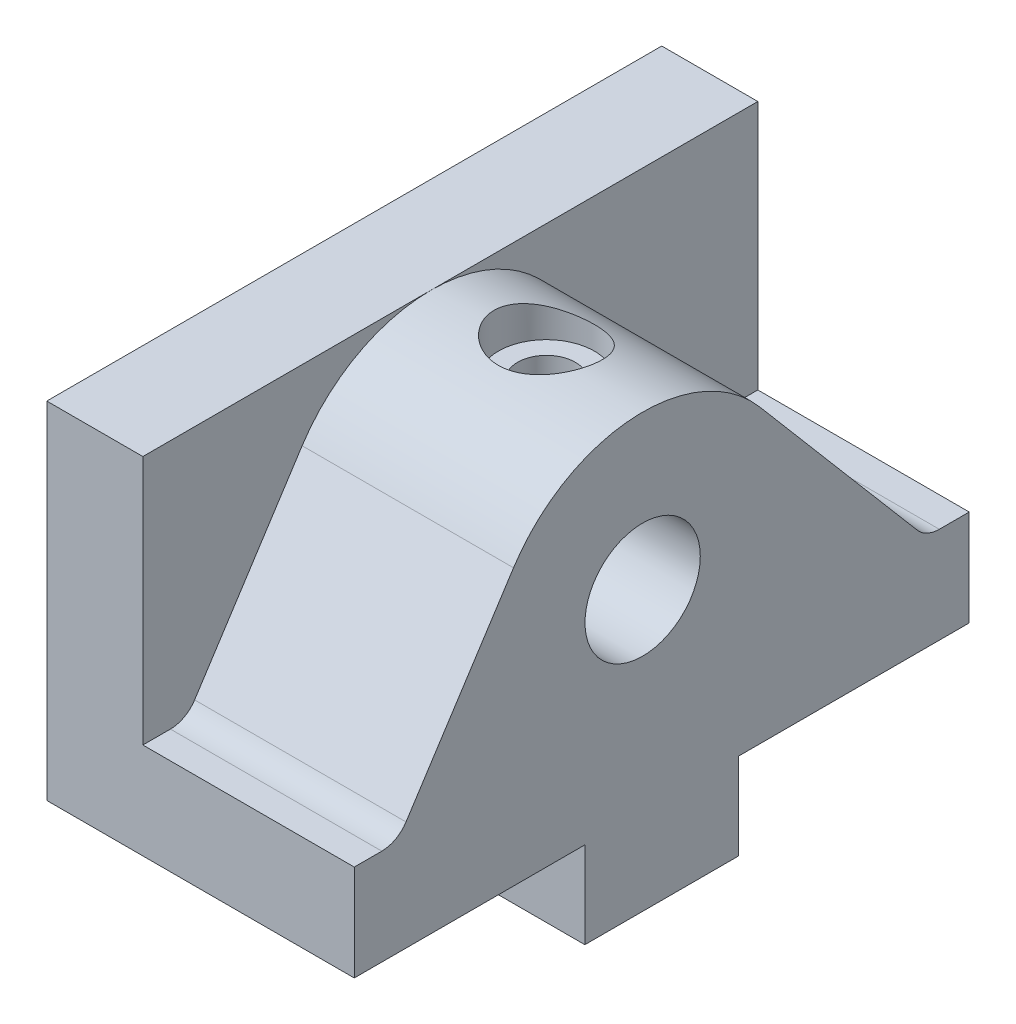
ISO-10303-21;
HEADER;
FILE_DESCRIPTION(('STEP AP214'),'2;1');
FILE_NAME('part.step','',(''),(''),'','','');
FILE_SCHEMA(('AUTOMOTIVE_DESIGN { 1 0 10303 214 1 1 1 1 }'));
ENDSEC;
DATA;
#1=APPLICATION_CONTEXT('core data for automotive mechanical design processes');
#2=APPLICATION_PROTOCOL_DEFINITION('international standard','automotive_design',2000,#1);
#3=PRODUCT_CONTEXT('',#1,'mechanical');
#4=PRODUCT('Part','Part','',(#3));
#5=PRODUCT_RELATED_PRODUCT_CATEGORY('part','',(#4));
#6=PRODUCT_DEFINITION_FORMATION('','',#4);
#7=PRODUCT_DEFINITION_CONTEXT('part definition',#1,'design');
#8=PRODUCT_DEFINITION('design','',#6,#7);
#9=PRODUCT_DEFINITION_SHAPE('','',#8);
#10=(LENGTH_UNIT() NAMED_UNIT(*) SI_UNIT(.MILLI.,.METRE.));
#11=(NAMED_UNIT(*) PLANE_ANGLE_UNIT() SI_UNIT($,.RADIAN.));
#12=(NAMED_UNIT(*) SI_UNIT($,.STERADIAN.) SOLID_ANGLE_UNIT());
#13=UNCERTAINTY_MEASURE_WITH_UNIT(LENGTH_MEASURE(1.E-05),#10,'distance_accuracy_value','');
#14=(GEOMETRIC_REPRESENTATION_CONTEXT(3) GLOBAL_UNCERTAINTY_ASSIGNED_CONTEXT((#13)) GLOBAL_UNIT_ASSIGNED_CONTEXT((#10,
#11,#12)) REPRESENTATION_CONTEXT('',''));
#15=CARTESIAN_POINT('',(0.,0.,0.));
#16=DIRECTION('',(0.,0.,1.));
#17=DIRECTION('',(1.,0.,0.));
#18=AXIS2_PLACEMENT_3D('',#15,#16,#17);
#19=CARTESIAN_POINT('',(0.,0.,-64.));
#20=DIRECTION('',(0.,-1.,0.));
#21=DIRECTION('',(0.,0.,-1.));
#22=AXIS2_PLACEMENT_3D('',#19,#20,#21);
#23=PLANE('',#22);
#24=DIRECTION('',(0.,0.,1.));
#25=VECTOR('',#24,1.);
#26=CARTESIAN_POINT('',(0.,0.,-64.));
#27=LINE('',#26,#25);
#28=CARTESIAN_POINT('',(0.,0.,-24.));
#29=VERTEX_POINT('',#28);
#30=CARTESIAN_POINT('',(0.,0.,0.));
#31=VERTEX_POINT('',#30);
#32=EDGE_CURVE('E244',#29,#31,#27,.T.);
#33=ORIENTED_EDGE('',*,*,#32,.F.);
#34=DIRECTION('',(1.,0.,0.));
#35=VECTOR('',#34,1.);
#36=CARTESIAN_POINT('',(-18.3575597506858,0.,-24.));
#37=LINE('',#36,#35);
#38=CARTESIAN_POINT('',(32.,0.,-24.));
#39=VERTEX_POINT('',#38);
#40=EDGE_CURVE('E192',#29,#39,#37,.T.);
#41=ORIENTED_EDGE('',*,*,#40,.T.);
#42=DIRECTION('',(0.,0.,1.));
#43=VECTOR('',#42,1.);
#44=CARTESIAN_POINT('',(32.,0.,-64.));
#45=LINE('',#44,#43);
#46=CARTESIAN_POINT('',(32.,0.,0.));
#47=VERTEX_POINT('',#46);
#48=EDGE_CURVE('E279',#39,#47,#45,.T.);
#49=ORIENTED_EDGE('',*,*,#48,.T.);
#50=DIRECTION('',(1.,0.,0.));
#51=VECTOR('',#50,1.);
#52=CARTESIAN_POINT('',(0.,0.,0.));
#53=LINE('',#52,#51);
#54=EDGE_CURVE('E247',#31,#47,#53,.T.);
#55=ORIENTED_EDGE('',*,*,#54,.F.);
#56=EDGE_LOOP('',(#33,#41,#49,#55));
#57=FACE_BOUND('',#56,.T.);
#58=ADVANCED_FACE('F39',(#57),#23,.T.);
#59=CARTESIAN_POINT('',(10.,10.,-64.));
#60=DIRECTION('',(1.,0.,0.));
#61=DIRECTION('',(0.,1.,0.));
#62=AXIS2_PLACEMENT_3D('',#59,#60,#61);
#63=PLANE('',#62);
#64=DIRECTION('',(0.,0.,1.));
#65=VECTOR('',#64,1.);
#66=CARTESIAN_POINT('',(10.,10.,-64.));
#67=LINE('',#66,#65);
#68=CARTESIAN_POINT('',(10.,10.,-2.86677840282892));
#69=VERTEX_POINT('',#68);
#70=CARTESIAN_POINT('',(10.,10.,0.));
#71=VERTEX_POINT('',#70);
#72=EDGE_CURVE('E269',#69,#71,#67,.T.);
#73=ORIENTED_EDGE('',*,*,#72,.F.);
#74=CARTESIAN_POINT('',(10.,13.,-2.86677840282891));
#75=DIRECTION('',(1.,0.,0.));
#76=DIRECTION('',(0.,1.,0.));
#77=AXIS2_PLACEMENT_3D('',#74,#75,#76);
#78=CIRCLE('',#77,3.);
#79=CARTESIAN_POINT('',(10.,11.3717245637124,-5.38644486956267));
#80=VERTEX_POINT('',#79);
#81=EDGE_CURVE('E288',#69,#80,#78,.T.);
#82=ORIENTED_EDGE('',*,*,#81,.T.);
#83=DIRECTION('',(0.,0.839888822244585,-0.542758478762518));
#84=VECTOR('',#83,1.);
#85=CARTESIAN_POINT('',(10.,10.,-4.5));
#86=LINE('',#85,#84);
#87=CARTESIAN_POINT('',(10.,28.6841356602003,-16.5741850341826));
#88=VERTEX_POINT('',#87);
#89=EDGE_CURVE('E210',#80,#88,#86,.T.);
#90=ORIENTED_EDGE('',*,*,#89,.T.);
#91=CARTESIAN_POINT('',(10.,20.,-30.012406190096));
#92=DIRECTION('',(1.,0.,0.));
#93=DIRECTION('',(0.,1.,0.));
#94=AXIS2_PLACEMENT_3D('',#91,#92,#93);
#95=CIRCLE('',#94,16.);
#96=CARTESIAN_POINT('',(10.,36.,-30.012406190096));
#97=VERTEX_POINT('',#96);
#98=EDGE_CURVE('E204',#88,#97,#95,.F.);
#99=ORIENTED_EDGE('',*,*,#98,.T.);
#100=DIRECTION('',(0.,0.,1.));
#101=VECTOR('',#100,1.);
#102=CARTESIAN_POINT('',(10.,36.,-64.));
#103=LINE('',#102,#101);
#104=CARTESIAN_POINT('',(10.,36.,0.));
#105=VERTEX_POINT('',#104);
#106=EDGE_CURVE('E266',#97,#105,#103,.T.);
#107=ORIENTED_EDGE('',*,*,#106,.T.);
#108=DIRECTION('',(0.,1.,0.));
#109=VECTOR('',#108,1.);
#110=CARTESIAN_POINT('',(10.,10.,0.));
#111=LINE('',#110,#109);
#112=EDGE_CURVE('E254',#71,#105,#111,.T.);
#113=ORIENTED_EDGE('',*,*,#112,.F.);
#114=EDGE_LOOP('',(#73,#82,#90,#99,#107,#113));
#115=FACE_BOUND('',#114,.T.);
#116=ADVANCED_FACE('F328',(#115),#63,.T.);
#117=CARTESIAN_POINT('',(32.,10.,-64.));
#118=DIRECTION('',(0.,1.,0.));
#119=DIRECTION('',(-1.,0.,0.));
#120=AXIS2_PLACEMENT_3D('',#117,#118,#119);
#121=PLANE('',#120);
#122=DIRECTION('',(0.,0.,1.));
#123=VECTOR('',#122,1.);
#124=CARTESIAN_POINT('',(32.,10.,-64.));
#125=LINE('',#124,#123);
#126=CARTESIAN_POINT('',(32.,10.,-2.86677840282892));
#127=VERTEX_POINT('',#126);
#128=CARTESIAN_POINT('',(32.,10.,0.));
#129=VERTEX_POINT('',#128);
#130=EDGE_CURVE('E273',#127,#129,#125,.T.);
#131=ORIENTED_EDGE('',*,*,#130,.F.);
#132=DIRECTION('',(1.,0.,0.));
#133=VECTOR('',#132,1.);
#134=CARTESIAN_POINT('',(10.,10.,-2.86677840282891));
#135=LINE('',#134,#133);
#136=EDGE_CURVE('E65',#127,#69,#135,.F.);
#137=ORIENTED_EDGE('',*,*,#136,.T.);
#138=ORIENTED_EDGE('',*,*,#72,.T.);
#139=DIRECTION('',(-1.,0.,0.));
#140=VECTOR('',#139,1.);
#141=CARTESIAN_POINT('',(32.,10.,0.));
#142=LINE('',#141,#140);
#143=EDGE_CURVE('E252',#129,#71,#142,.T.);
#144=ORIENTED_EDGE('',*,*,#143,.F.);
#145=EDGE_LOOP('',(#131,#137,#138,#144));
#146=FACE_BOUND('',#145,.T.);
#147=ADVANCED_FACE('F357',(#146),#121,.T.);
#148=CARTESIAN_POINT('',(0.,36.,-64.));
#149=DIRECTION('',(-1.,0.,0.));
#150=DIRECTION('',(0.,0.,1.));
#151=AXIS2_PLACEMENT_3D('',#148,#149,#150);
#152=PLANE('',#151);
#153=CARTESIAN_POINT('',(0.,20.,-30.012406190096));
#154=DIRECTION('',(-1.,0.,0.));
#155=DIRECTION('',(0.,0.,1.));
#156=AXIS2_PLACEMENT_3D('',#153,#154,#155);
#157=CIRCLE('',#156,5.99999999999999);
#158=CARTESIAN_POINT('',(0.,20.,-24.012406190096));
#159=VERTEX_POINT('',#158);
#160=EDGE_CURVE('E199',#159,#159,#157,.F.);
#161=ORIENTED_EDGE('',*,*,#160,.T.);
#162=EDGE_LOOP('',(#161));
#163=FACE_BOUND('',#162,.T.);
#164=DIRECTION('',(0.,-1.,0.));
#165=VECTOR('',#164,1.);
#166=CARTESIAN_POINT('',(0.,36.,0.));
#167=LINE('',#166,#165);
#168=CARTESIAN_POINT('',(0.,36.,0.));
#169=VERTEX_POINT('',#168);
#170=EDGE_CURVE('E221',#169,#31,#167,.T.);
#171=ORIENTED_EDGE('',*,*,#170,.F.);
#172=DIRECTION('',(0.,0.,1.));
#173=VECTOR('',#172,1.);
#174=CARTESIAN_POINT('',(0.,36.,-64.));
#175=LINE('',#174,#173);
#176=CARTESIAN_POINT('',(0.,36.,-64.));
#177=VERTEX_POINT('',#176);
#178=EDGE_CURVE('E257',#177,#169,#175,.T.);
#179=ORIENTED_EDGE('',*,*,#178,.F.);
#180=DIRECTION('',(0.,-1.,0.));
#181=VECTOR('',#180,1.);
#182=CARTESIAN_POINT('',(0.,36.,-64.));
#183=LINE('',#182,#181);
#184=CARTESIAN_POINT('',(0.,0.,-64.));
#185=VERTEX_POINT('',#184);
#186=EDGE_CURVE('E223',#177,#185,#183,.T.);
#187=ORIENTED_EDGE('',*,*,#186,.T.);
#188=CARTESIAN_POINT('',(0.,0.,-40.));
#189=VERTEX_POINT('',#188);
#190=EDGE_CURVE('E167',#185,#189,#27,.T.);
#191=ORIENTED_EDGE('',*,*,#190,.T.);
#192=DIRECTION('',(0.,1.,0.));
#193=VECTOR('',#192,1.);
#194=CARTESIAN_POINT('',(0.,0.,-40.));
#195=LINE('',#194,#193);
#196=CARTESIAN_POINT('',(0.,-9.,-40.));
#197=VERTEX_POINT('',#196);
#198=EDGE_CURVE('E158',#197,#189,#195,.T.);
#199=ORIENTED_EDGE('',*,*,#198,.F.);
#200=DIRECTION('',(0.,0.,-1.));
#201=VECTOR('',#200,1.);
#202=CARTESIAN_POINT('',(0.,-9.,-24.));
#203=LINE('',#202,#201);
#204=CARTESIAN_POINT('',(0.,-9.,-24.));
#205=VERTEX_POINT('',#204);
#206=EDGE_CURVE('E162',#205,#197,#203,.T.);
#207=ORIENTED_EDGE('',*,*,#206,.F.);
#208=DIRECTION('',(0.,-1.,0.));
#209=VECTOR('',#208,1.);
#210=CARTESIAN_POINT('',(0.,0.,-24.));
#211=LINE('',#210,#209);
#212=EDGE_CURVE('E190',#29,#205,#211,.T.);
#213=ORIENTED_EDGE('',*,*,#212,.F.);
#214=ORIENTED_EDGE('',*,*,#32,.T.);
#215=EDGE_LOOP('',(#171,#179,#187,#191,#199,#207,#213,#214));
#216=FACE_BOUND('',#215,.T.);
#217=ADVANCED_FACE('F161',(#163,#216),#152,.T.);
#218=CARTESIAN_POINT('',(10.,36.,-64.));
#219=DIRECTION('',(0.,1.,0.));
#220=DIRECTION('',(0.,0.,1.));
#221=AXIS2_PLACEMENT_3D('',#218,#219,#220);
#222=PLANE('',#221);
#223=DIRECTION('',(-1.,0.,0.));
#224=VECTOR('',#223,1.);
#225=CARTESIAN_POINT('',(10.,36.,0.));
#226=LINE('',#225,#224);
#227=EDGE_CURVE('E229',#105,#169,#226,.T.);
#228=ORIENTED_EDGE('',*,*,#227,.F.);
#229=ORIENTED_EDGE('',*,*,#106,.F.);
#230=CARTESIAN_POINT('',(10.,36.,-64.));
#231=VERTEX_POINT('',#230);
#232=EDGE_CURVE('E263',#231,#97,#103,.T.);
#233=ORIENTED_EDGE('',*,*,#232,.F.);
#234=DIRECTION('',(-1.,0.,0.));
#235=VECTOR('',#234,1.);
#236=CARTESIAN_POINT('',(10.,36.,-64.));
#237=LINE('',#236,#235);
#238=EDGE_CURVE('E238',#231,#177,#237,.T.);
#239=ORIENTED_EDGE('',*,*,#238,.T.);
#240=ORIENTED_EDGE('',*,*,#178,.T.);
#241=EDGE_LOOP('',(#228,#229,#233,#239,#240));
#242=FACE_BOUND('',#241,.T.);
#243=ADVANCED_FACE('F325',(#242),#222,.T.);
#244=DIRECTION('',(0.,-0.762150851836937,-0.647399474083993));
#245=VECTOR('',#244,1.);
#246=CARTESIAN_POINT('',(10.,30.3583915853439,-42.206819819487));
#247=LINE('',#246,#245);
#248=CARTESIAN_POINT('',(10.,30.3583915853439,-42.206819819487));
#249=VERTEX_POINT('',#248);
#250=CARTESIAN_POINT('',(10.,11.057801577748,-58.6014637279894));
#251=VERTEX_POINT('',#250);
#252=EDGE_CURVE('E209',#249,#251,#247,.T.);
#253=ORIENTED_EDGE('',*,*,#252,.T.);
#254=CARTESIAN_POINT('',(10.,13.,-60.8879162835002));
#255=DIRECTION('',(1.,0.,0.));
#256=DIRECTION('',(0.,1.,0.));
#257=AXIS2_PLACEMENT_3D('',#254,#255,#256);
#258=CIRCLE('',#257,3.);
#259=CARTESIAN_POINT('',(10.,10.,-60.8879162835002));
#260=VERTEX_POINT('',#259);
#261=EDGE_CURVE('E283',#251,#260,#258,.T.);
#262=ORIENTED_EDGE('',*,*,#261,.T.);
#263=CARTESIAN_POINT('',(10.,10.,-64.));
#264=VERTEX_POINT('',#263);
#265=EDGE_CURVE('E270',#264,#260,#67,.T.);
#266=ORIENTED_EDGE('',*,*,#265,.F.);
#267=DIRECTION('',(0.,1.,0.));
#268=VECTOR('',#267,1.);
#269=CARTESIAN_POINT('',(10.,10.,-64.));
#270=LINE('',#269,#268);
#271=EDGE_CURVE('E240',#264,#231,#270,.T.);
#272=ORIENTED_EDGE('',*,*,#271,.T.);
#273=ORIENTED_EDGE('',*,*,#232,.T.);
#274=EDGE_CURVE('E208',#97,#249,#95,.F.);
#275=ORIENTED_EDGE('',*,*,#274,.T.);
#276=EDGE_LOOP('',(#253,#262,#266,#272,#273,#275));
#277=FACE_BOUND('',#276,.T.);
#278=ADVANCED_FACE('F308',(#277),#63,.T.);
#279=ORIENTED_EDGE('',*,*,#265,.T.);
#280=DIRECTION('',(1.,0.,0.));
#281=VECTOR('',#280,1.);
#282=CARTESIAN_POINT('',(32.,10.,-60.8879162835002));
#283=LINE('',#282,#281);
#284=CARTESIAN_POINT('',(32.,10.,-60.8879162835002));
#285=VERTEX_POINT('',#284);
#286=EDGE_CURVE('E265',#260,#285,#283,.T.);
#287=ORIENTED_EDGE('',*,*,#286,.T.);
#288=CARTESIAN_POINT('',(32.,10.,-64.));
#289=VERTEX_POINT('',#288);
#290=EDGE_CURVE('E271',#289,#285,#125,.T.);
#291=ORIENTED_EDGE('',*,*,#290,.F.);
#292=DIRECTION('',(-1.,0.,0.));
#293=VECTOR('',#292,1.);
#294=CARTESIAN_POINT('',(32.,10.,-64.));
#295=LINE('',#294,#293);
#296=EDGE_CURVE('E231',#289,#264,#295,.T.);
#297=ORIENTED_EDGE('',*,*,#296,.T.);
#298=EDGE_LOOP('',(#279,#287,#291,#297));
#299=FACE_BOUND('',#298,.T.);
#300=ADVANCED_FACE('F309',(#299),#121,.T.);
#301=CARTESIAN_POINT('',(32.,0.,-64.));
#302=DIRECTION('',(1.,0.,0.));
#303=DIRECTION('',(0.,0.,-1.));
#304=AXIS2_PLACEMENT_3D('',#301,#302,#303);
#305=PLANE('',#304);
#306=CARTESIAN_POINT('',(32.,20.,-30.012406190096));
#307=DIRECTION('',(1.,0.,0.));
#308=DIRECTION('',(0.,0.,-1.));
#309=AXIS2_PLACEMENT_3D('',#306,#307,#308);
#310=CIRCLE('',#309,5.99999999999999);
#311=CARTESIAN_POINT('',(32.,20.,-36.012406190096));
#312=VERTEX_POINT('',#311);
#313=EDGE_CURVE('E197',#312,#312,#310,.T.);
#314=ORIENTED_EDGE('',*,*,#313,.F.);
#315=EDGE_LOOP('',(#314));
#316=FACE_BOUND('',#315,.T.);
#317=DIRECTION('',(0.,1.,0.));
#318=VECTOR('',#317,1.);
#319=CARTESIAN_POINT('',(32.,0.,0.));
#320=LINE('',#319,#318);
#321=EDGE_CURVE('E246',#47,#129,#320,.T.);
#322=ORIENTED_EDGE('',*,*,#321,.F.);
#323=ORIENTED_EDGE('',*,*,#48,.F.);
#324=DIRECTION('',(0.,-1.,0.));
#325=VECTOR('',#324,1.);
#326=CARTESIAN_POINT('',(32.,0.,-24.));
#327=LINE('',#326,#325);
#328=CARTESIAN_POINT('',(32.,-9.,-24.));
#329=VERTEX_POINT('',#328);
#330=EDGE_CURVE('E189',#39,#329,#327,.T.);
#331=ORIENTED_EDGE('',*,*,#330,.T.);
#332=DIRECTION('',(0.,0.,-1.));
#333=VECTOR('',#332,1.);
#334=CARTESIAN_POINT('',(32.,-9.,-24.));
#335=LINE('',#334,#333);
#336=CARTESIAN_POINT('',(32.,-9.,-40.));
#337=VERTEX_POINT('',#336);
#338=EDGE_CURVE('E184',#329,#337,#335,.T.);
#339=ORIENTED_EDGE('',*,*,#338,.T.);
#340=DIRECTION('',(0.,1.,0.));
#341=VECTOR('',#340,1.);
#342=CARTESIAN_POINT('',(32.,0.,-40.));
#343=LINE('',#342,#341);
#344=CARTESIAN_POINT('',(32.,0.,-40.));
#345=VERTEX_POINT('',#344);
#346=EDGE_CURVE('E175',#337,#345,#343,.T.);
#347=ORIENTED_EDGE('',*,*,#346,.T.);
#348=CARTESIAN_POINT('',(32.,0.,-64.));
#349=VERTEX_POINT('',#348);
#350=EDGE_CURVE('E274',#349,#345,#45,.T.);
#351=ORIENTED_EDGE('',*,*,#350,.F.);
#352=DIRECTION('',(0.,1.,0.));
#353=VECTOR('',#352,1.);
#354=CARTESIAN_POINT('',(32.,0.,-64.));
#355=LINE('',#354,#353);
#356=EDGE_CURVE('E232',#349,#289,#355,.T.);
#357=ORIENTED_EDGE('',*,*,#356,.T.);
#358=ORIENTED_EDGE('',*,*,#290,.T.);
#359=CARTESIAN_POINT('',(32.,13.,-60.8879162835002));
#360=DIRECTION('',(1.,0.,0.));
#361=DIRECTION('',(0.,0.,-1.));
#362=AXIS2_PLACEMENT_3D('',#359,#360,#361);
#363=CIRCLE('',#362,3.);
#364=CARTESIAN_POINT('',(32.,11.057801577748,-58.6014637279894));
#365=VERTEX_POINT('',#364);
#366=EDGE_CURVE('E295',#285,#365,#363,.F.);
#367=ORIENTED_EDGE('',*,*,#366,.T.);
#368=DIRECTION('',(0.,0.762150851836937,0.647399474083993));
#369=VECTOR('',#368,1.);
#370=CARTESIAN_POINT('',(32.,30.3583915853439,-42.206819819487));
#371=LINE('',#370,#369);
#372=CARTESIAN_POINT('',(32.,30.3583915853439,-42.206819819487));
#373=VERTEX_POINT('',#372);
#374=EDGE_CURVE('E201',#365,#373,#371,.T.);
#375=ORIENTED_EDGE('',*,*,#374,.T.);
#376=CARTESIAN_POINT('',(32.,20.,-30.012406190096));
#377=DIRECTION('',(1.,0.,0.));
#378=DIRECTION('',(0.,0.,1.));
#379=AXIS2_PLACEMENT_3D('',#376,#377,#378);
#380=CIRCLE('',#379,16.);
#381=CARTESIAN_POINT('',(32.,28.6841356602003,-16.5741850341826));
#382=VERTEX_POINT('',#381);
#383=EDGE_CURVE('E215',#373,#382,#380,.T.);
#384=ORIENTED_EDGE('',*,*,#383,.T.);
#385=DIRECTION('',(0.,-0.839888822244585,0.542758478762518));
#386=VECTOR('',#385,1.);
#387=CARTESIAN_POINT('',(32.,10.,-4.5));
#388=LINE('',#387,#386);
#389=CARTESIAN_POINT('',(32.,11.3717245637124,-5.38644486956267));
#390=VERTEX_POINT('',#389);
#391=EDGE_CURVE('E214',#382,#390,#388,.T.);
#392=ORIENTED_EDGE('',*,*,#391,.T.);
#393=CARTESIAN_POINT('',(32.,13.,-2.86677840282892));
#394=DIRECTION('',(1.,0.,0.));
#395=DIRECTION('',(0.,0.,-1.));
#396=AXIS2_PLACEMENT_3D('',#393,#394,#395);
#397=CIRCLE('',#396,3.);
#398=EDGE_CURVE('E55',#390,#127,#397,.F.);
#399=ORIENTED_EDGE('',*,*,#398,.T.);
#400=ORIENTED_EDGE('',*,*,#130,.T.);
#401=EDGE_LOOP('',(#322,#323,#331,#339,#347,#351,#357,#358,#367,#375,#384,#392,#399,#400));
#402=FACE_BOUND('',#401,.T.);
#403=ADVANCED_FACE('F293',(#316,#402),#305,.T.);
#404=DIRECTION('',(1.,0.,0.));
#405=VECTOR('',#404,1.);
#406=CARTESIAN_POINT('',(-18.3575597506858,0.,-40.));
#407=LINE('',#406,#405);
#408=EDGE_CURVE('E166',#189,#345,#407,.T.);
#409=ORIENTED_EDGE('',*,*,#408,.F.);
#410=ORIENTED_EDGE('',*,*,#190,.F.);
#411=DIRECTION('',(1.,0.,0.));
#412=VECTOR('',#411,1.);
#413=CARTESIAN_POINT('',(0.,0.,-64.));
#414=LINE('',#413,#412);
#415=EDGE_CURVE('E227',#185,#349,#414,.T.);
#416=ORIENTED_EDGE('',*,*,#415,.T.);
#417=ORIENTED_EDGE('',*,*,#350,.T.);
#418=EDGE_LOOP('',(#409,#410,#416,#417));
#419=FACE_BOUND('',#418,.T.);
#420=ADVANCED_FACE('F317',(#419),#23,.T.);
#421=CARTESIAN_POINT('',(0.,0.,-64.));
#422=DIRECTION('',(0.,0.,1.));
#423=DIRECTION('',(1.,0.,0.));
#424=AXIS2_PLACEMENT_3D('',#421,#422,#423);
#425=PLANE('',#424);
#426=ORIENTED_EDGE('',*,*,#186,.F.);
#427=ORIENTED_EDGE('',*,*,#238,.F.);
#428=ORIENTED_EDGE('',*,*,#271,.F.);
#429=ORIENTED_EDGE('',*,*,#296,.F.);
#430=ORIENTED_EDGE('',*,*,#356,.F.);
#431=ORIENTED_EDGE('',*,*,#415,.F.);
#432=EDGE_LOOP('',(#426,#427,#428,#429,#430,#431));
#433=FACE_BOUND('',#432,.T.);
#434=ADVANCED_FACE('F312',(#433),#425,.F.);
#435=CARTESIAN_POINT('',(0.,0.,0.));
#436=DIRECTION('',(0.,0.,1.));
#437=DIRECTION('',(1.,0.,0.));
#438=AXIS2_PLACEMENT_3D('',#435,#436,#437);
#439=PLANE('',#438);
#440=ORIENTED_EDGE('',*,*,#170,.T.);
#441=ORIENTED_EDGE('',*,*,#54,.T.);
#442=ORIENTED_EDGE('',*,*,#321,.T.);
#443=ORIENTED_EDGE('',*,*,#143,.T.);
#444=ORIENTED_EDGE('',*,*,#112,.T.);
#445=ORIENTED_EDGE('',*,*,#227,.T.);
#446=EDGE_LOOP('',(#440,#441,#442,#443,#444,#445));
#447=FACE_BOUND('',#446,.T.);
#448=ADVANCED_FACE('F368',(#447),#439,.T.);
#449=CARTESIAN_POINT('',(-50.8358446970205,10.,-4.5));
#450=DIRECTION('',(0.,0.542758478762518,0.839888822244585));
#451=DIRECTION('',(0.,-0.839888822244585,0.542758478762518));
#452=AXIS2_PLACEMENT_3D('',#449,#450,#451);
#453=PLANE('',#452);
#454=ORIENTED_EDGE('',*,*,#89,.F.);
#455=DIRECTION('',(1.,0.,0.));
#456=VECTOR('',#455,1.);
#457=CARTESIAN_POINT('',(32.,11.3717245637124,-5.38644486956267));
#458=LINE('',#457,#456);
#459=EDGE_CURVE('E287',#80,#390,#458,.T.);
#460=ORIENTED_EDGE('',*,*,#459,.T.);
#461=ORIENTED_EDGE('',*,*,#391,.F.);
#462=DIRECTION('',(1.,0.,0.));
#463=VECTOR('',#462,1.);
#464=CARTESIAN_POINT('',(-50.8358446970205,28.6841356602003,-16.5741850341826));
#465=LINE('',#464,#463);
#466=EDGE_CURVE('E217',#88,#382,#465,.T.);
#467=ORIENTED_EDGE('',*,*,#466,.F.);
#468=EDGE_LOOP('',(#454,#460,#461,#467));
#469=FACE_BOUND('',#468,.T.);
#470=ADVANCED_FACE('F333',(#469),#453,.T.);
#471=CARTESIAN_POINT('',(-50.8358446970205,20.,-30.012406190096));
#472=DIRECTION('',(1.,0.,0.));
#473=DIRECTION('',(0.,0.,-1.));
#474=AXIS2_PLACEMENT_3D('',#471,#472,#473);
#475=CYLINDRICAL_SURFACE('',#474,16.);
#476=CARTESIAN_POINT('',(20.,35.7138604087561,-27.));
#477=CARTESIAN_POINT('',(20.278848664768,35.7138621416898,-27.0000024118392));
#478=CARTESIAN_POINT('',(20.5577209979948,35.7183995053292,-27.023393326629));
#479=CARTESIAN_POINT('',(21.1074555341942,35.7357648435869,-27.1162219379741));
#480=CARTESIAN_POINT('',(21.3783160093169,35.7485945931165,-27.1856694926263));
#481=CARTESIAN_POINT('',(21.9041778362452,35.7802998697871,-27.3684195303028));
#482=CARTESIAN_POINT('',(22.1591912253849,35.7991707394135,-27.4816882425671));
#483=CARTESIAN_POINT('',(22.6467236044746,35.8396517240156,-27.7488657856995));
#484=CARTESIAN_POINT('',(22.8792406328494,35.8612620774823,-27.9027781561446));
#485=CARTESIAN_POINT('',(23.3181501647711,35.9035094129234,-28.249141970418));
#486=CARTESIAN_POINT('',(23.5242049832579,35.9241320388914,-28.442023472432));
#487=CARTESIAN_POINT('',(23.9011989312148,35.9598172549529,-28.8599636350324));
#488=CARTESIAN_POINT('',(24.0721398358305,35.9748801261444,-29.0850206680437));
#489=CARTESIAN_POINT('',(24.3731133348381,35.9953511562227,-29.5598228331938));
#490=CARTESIAN_POINT('',(24.5033508535935,36.0008083414371,-29.8094356935987));
#491=CARTESIAN_POINT('',(24.7201072533691,35.9989972876808,-30.3269105215898));
#492=CARTESIAN_POINT('',(24.8066368375074,35.9917321660733,-30.5947680032166));
#493=CARTESIAN_POINT('',(24.9316332640666,35.9629599633376,-31.132312445951));
#494=CARTESIAN_POINT('',(24.9714497426838,35.9418817640369,-31.4017094168431));
#495=CARTESIAN_POINT('',(25.0069841502588,35.8855533972796,-31.9418935644978));
#496=CARTESIAN_POINT('',(25.0027037349677,35.85030376198,-32.2126806886814));
#497=CARTESIAN_POINT('',(24.9511743967235,35.7669470586088,-32.7466480726776));
#498=CARTESIAN_POINT('',(24.9041405870106,35.7189052092163,-33.0098596157745));
#499=CARTESIAN_POINT('',(24.7696524512278,35.61221801056,-33.5234639476529));
#500=CARTESIAN_POINT('',(24.6821898118877,35.5535704819898,-33.7738540882362));
#501=CARTESIAN_POINT('',(24.4650143999639,35.4261425808312,-34.2670361372327));
#502=CARTESIAN_POINT('',(24.3335826138006,35.3570257170226,-34.5089835749196));
#503=CARTESIAN_POINT('',(24.0335263814342,35.2152914427282,-34.9674648317593));
#504=CARTESIAN_POINT('',(23.864886780741,35.1426726153609,-35.1839882406624));
#505=CARTESIAN_POINT('',(23.4840704371725,34.9951275877623,-35.5978278096722));
#506=CARTESIAN_POINT('',(23.270043540879,34.920286571019,-35.7934906354605));
#507=CARTESIAN_POINT('',(22.9250231163291,34.8142809839663,-36.0577480084317));
#508=CARTESIAN_POINT('',(22.8059399465649,34.7799694965151,-36.1410026826001));
#509=CARTESIAN_POINT('',(22.5604201780935,34.7142560069259,-36.2971356810007));
#510=CARTESIAN_POINT('',(22.4339870470747,34.6828526505861,-36.3700188434081));
#511=CARTESIAN_POINT('',(22.1763727507677,34.6241966943476,-36.5037958131474));
#512=CARTESIAN_POINT('',(22.0452838101075,34.5968917566604,-36.564844349114));
#513=CARTESIAN_POINT('',(21.7776363928718,34.5466809580857,-36.6755712872092));
#514=CARTESIAN_POINT('',(21.6410805108573,34.5237730396351,-36.7252550095422));
#515=CARTESIAN_POINT('',(21.3635325714462,34.4830430698752,-36.8126850317504));
#516=CARTESIAN_POINT('',(21.2225428247084,34.4652184166913,-36.850437439756));
#517=CARTESIAN_POINT('',(20.9372286120054,34.4352168373357,-36.9135467543385));
#518=CARTESIAN_POINT('',(20.7929044932603,34.423039325865,-36.9389049455308));
#519=CARTESIAN_POINT('',(20.5153273628942,34.405568692793,-36.9751609818758));
#520=CARTESIAN_POINT('',(20.3822495013769,34.399753820978,-36.9871565291217));
#521=CARTESIAN_POINT('',(20.1154379388309,34.3933069292877,-37.0004511530126));
#522=CARTESIAN_POINT('',(19.981704276963,34.3926746036208,-37.0017508607563));
#523=CARTESIAN_POINT('',(19.7146664993111,34.3966112104088,-36.9936385411063));
#524=CARTESIAN_POINT('',(19.5813623067823,34.4011791552128,-36.9842285477308));
#525=CARTESIAN_POINT('',(19.3162046786125,34.4153802212201,-36.9548177570351));
#526=CARTESIAN_POINT('',(19.1843512290668,34.4250132938338,-36.9348170613112));
#527=CARTESIAN_POINT('',(18.9296036378895,34.4484707533361,-36.8857164356188));
#528=CARTESIAN_POINT('',(18.8065906807948,34.4620620837967,-36.8571201944255));
#529=CARTESIAN_POINT('',(18.5635326893385,34.4932306627892,-36.7908717689638));
#530=CARTESIAN_POINT('',(18.4434886258924,34.5108091966272,-36.7532166642622));
#531=CARTESIAN_POINT('',(18.0889489982007,34.568924212728,-36.6271678832958));
#532=CARTESIAN_POINT('',(17.8598542986359,34.6148587093208,-36.5256532815535));
#533=CARTESIAN_POINT('',(17.4089331874678,34.7200931975071,-36.2843316960081));
#534=CARTESIAN_POINT('',(17.1882400310301,34.7799995454241,-36.1426923351535));
#535=CARTESIAN_POINT('',(16.7727566338718,34.9066674370778,-35.8279060574763));
#536=CARTESIAN_POINT('',(16.5779777489062,34.9734319635398,-35.6547454060739));
#537=CARTESIAN_POINT('',(16.2018841746903,35.115117201762,-35.2640794466606));
#538=CARTESIAN_POINT('',(16.0233112929487,35.1902349218076,-35.0439988870224));
#539=CARTESIAN_POINT('',(15.705386674332,35.3373000170745,-34.5761045541109));
#540=CARTESIAN_POINT('',(15.5660434036009,35.4092467051339,-34.3282848105459));
#541=CARTESIAN_POINT('',(15.3279322075799,35.5465270855229,-33.8045546943471));
#542=CARTESIAN_POINT('',(15.2301976907428,35.6116650171455,-33.5281200272475));
#543=CARTESIAN_POINT('',(15.0842401388742,35.7288499337635,-32.9598280262817));
#544=CARTESIAN_POINT('',(15.035997849133,35.7809020037948,-32.6679767366788));
#545=CARTESIAN_POINT('',(14.9929739412356,35.8666987674266,-32.092824124224));
#546=CARTESIAN_POINT('',(14.9956192901381,35.9012342434611,-31.8098337295577));
#547=CARTESIAN_POINT('',(15.0489627707916,35.9548034787661,-31.246951717227));
#548=CARTESIAN_POINT('',(15.0996475115444,35.9738415551935,-30.9670592580071));
#549=CARTESIAN_POINT('',(15.2444807844625,35.9966336704063,-30.4321120839769));
#550=CARTESIAN_POINT('',(15.3365067780703,36.001054973073,-30.1765074184742));
#551=CARTESIAN_POINT('',(15.5606678003013,35.998521241655,-29.6836170588233));
#552=CARTESIAN_POINT('',(15.6928039944006,35.9915658769745,-29.4463318972337));
#553=CARTESIAN_POINT('',(15.9943326581648,35.9692429400062,-28.9952235651992));
#554=CARTESIAN_POINT('',(16.1639381150947,35.953826496958,-28.7815454447151));
#555=CARTESIAN_POINT('',(16.5353572880085,35.9182427743642,-28.384735772739));
#556=CARTESIAN_POINT('',(16.7371776248496,35.8980745178112,-28.2016105163816));
#557=CARTESIAN_POINT('',(17.1742040801057,35.8562573842161,-27.8656225163763));
#558=CARTESIAN_POINT('',(17.4102237150583,35.8345823231938,-27.7138200687168));
#559=CARTESIAN_POINT('',(17.9044875337429,35.7943168008869,-27.4516980944413));
#560=CARTESIAN_POINT('',(18.1627279717011,35.7757258212579,-27.3413715929699));
#561=CARTESIAN_POINT('',(18.6812352110359,35.7456758120055,-27.1697074363759));
#562=CARTESIAN_POINT('',(18.9407748820014,35.7339104434347,-27.1062233611347));
#563=CARTESIAN_POINT('',(19.4668695959251,35.7180022687967,-27.0213704532717));
#564=CARTESIAN_POINT('',(19.7334239825025,35.713858752092,-26.9999976943103));
#565=CARTESIAN_POINT('',(20.,35.7138604087561,-27.));
#566=B_SPLINE_CURVE_WITH_KNOTS('',3,(#476,#477,#478,#479,#480,#481,#482,#483,#484,#485,#486,
#487,#488,#489,#490,#491,#492,#493,#494,#495,#496,#497,#498,#499,#500,#501,#502,#503,#504,#505,
#506,#507,#508,#509,#510,#511,#512,#513,#514,#515,#516,#517,#518,#519,#520,#521,#522,#523,#524,
#525,#526,#527,#528,#529,#530,#531,#532,#533,#534,#535,#536,#537,#538,#539,#540,#541,#542,#543,
#544,#545,#546,#547,#548,#549,#550,#551,#552,#553,#554,#555,#556,#557,#558,#559,#560,#561,#562,
#563,#564,#565),.UNSPECIFIED.,.T.,.F.,(4,2,2,2,2,2,2,2,2,2,2,2,2,2,2,2,2,2,2,2,2,2,2,2,2,2,2,2,
2,2,2,2,2,2,2,2,2,2,2,2,2,2,2,2,4),(0.,0.835584483785956,1.67134787624966,2.50646846682765,
3.34166181042866,4.18663217765951,5.03155981781443,5.87216240097696,6.71255903902033,
7.52802527056166,8.3434608830723,9.15481621415704,9.96633845630042,10.8142581354797,
11.6625238062088,12.5562917588331,13.0037199433121,13.4509387193141,13.8918441181281,
14.332542691779,14.7730152868715,15.2134422188945,15.6141562672501,16.0148466716529,
16.4154609884419,16.8160714622177,17.1966974291035,17.5774462685598,18.3383621465955,
19.1420690409361,19.9461269714857,20.8217569241029,21.6975757018499,22.5940307679908,
23.4901369402506,24.3410580041048,25.1917419431334,26.0030124962317,26.8143066245545,
27.6303368296247,28.4465349630692,29.2869735145374,30.1272706692938,30.9261540182756,
31.7249628781124),.UNSPECIFIED.);
#567=CARTESIAN_POINT('',(20.,35.7138604087561,-27.));
#568=VERTEX_POINT('',#567);
#569=EDGE_CURVE('E11',#568,#568,#566,.T.);
#570=ORIENTED_EDGE('',*,*,#569,.F.);
#571=EDGE_LOOP('',(#570));
#572=FACE_BOUND('',#571,.T.);
#573=ORIENTED_EDGE('',*,*,#98,.F.);
#574=ORIENTED_EDGE('',*,*,#466,.T.);
#575=ORIENTED_EDGE('',*,*,#383,.F.);
#576=DIRECTION('',(1.,0.,0.));
#577=VECTOR('',#576,1.);
#578=CARTESIAN_POINT('',(-50.8358446970205,30.3583915853439,-42.206819819487));
#579=LINE('',#578,#577);
#580=EDGE_CURVE('E220',#249,#373,#579,.T.);
#581=ORIENTED_EDGE('',*,*,#580,.F.);
#582=ORIENTED_EDGE('',*,*,#274,.F.);
#583=EDGE_LOOP('',(#573,#574,#575,#581,#582));
#584=FACE_BOUND('',#583,.T.);
#585=ADVANCED_FACE('F326',(#572,#584),#475,.T.);
#586=CARTESIAN_POINT('',(-50.8358446970205,30.3583915853439,-42.206819819487));
#587=DIRECTION('',(0.,0.647399474083993,-0.762150851836937));
#588=DIRECTION('',(0.,0.762150851836937,0.647399474083993));
#589=AXIS2_PLACEMENT_3D('',#586,#587,#588);
#590=PLANE('',#589);
#591=ORIENTED_EDGE('',*,*,#374,.F.);
#592=DIRECTION('',(1.,0.,0.));
#593=VECTOR('',#592,1.);
#594=CARTESIAN_POINT('',(10.,11.057801577748,-58.6014637279894));
#595=LINE('',#594,#593);
#596=EDGE_CURVE('E282',#365,#251,#595,.F.);
#597=ORIENTED_EDGE('',*,*,#596,.T.);
#598=ORIENTED_EDGE('',*,*,#252,.F.);
#599=ORIENTED_EDGE('',*,*,#580,.T.);
#600=EDGE_LOOP('',(#591,#597,#598,#599));
#601=FACE_BOUND('',#600,.T.);
#602=ADVANCED_FACE('F300',(#601),#590,.T.);
#603=CARTESIAN_POINT('',(-16.9705627484771,20.,-30.012406190096));
#604=DIRECTION('',(1.,0.,0.));
#605=DIRECTION('',(0.,0.,-1.));
#606=AXIS2_PLACEMENT_3D('',#603,#604,#605);
#607=CYLINDRICAL_SURFACE('',#606,5.99999999999999);
#608=ORIENTED_EDGE('',*,*,#313,.T.);
#609=EDGE_LOOP('',(#608));
#610=FACE_BOUND('',#609,.T.);
#611=ORIENTED_EDGE('',*,*,#160,.F.);
#612=EDGE_LOOP('',(#611));
#613=FACE_BOUND('',#612,.T.);
#614=ADVANCED_FACE('F383',(#610,#613),#607,.F.);
#615=CARTESIAN_POINT('',(-18.3575597506858,-9.,-24.));
#616=DIRECTION('',(0.,-1.,0.));
#617=DIRECTION('',(0.,0.,-1.));
#618=AXIS2_PLACEMENT_3D('',#615,#616,#617);
#619=PLANE('',#618);
#620=DIRECTION('',(1.,0.,0.));
#621=VECTOR('',#620,1.);
#622=CARTESIAN_POINT('',(-18.3575597506858,-9.,-24.));
#623=LINE('',#622,#621);
#624=EDGE_CURVE('E185',#205,#329,#623,.T.);
#625=ORIENTED_EDGE('',*,*,#624,.F.);
#626=ORIENTED_EDGE('',*,*,#206,.T.);
#627=DIRECTION('',(1.,0.,0.));
#628=VECTOR('',#627,1.);
#629=CARTESIAN_POINT('',(-18.3575597506858,-9.,-40.));
#630=LINE('',#629,#628);
#631=EDGE_CURVE('E168',#197,#337,#630,.T.);
#632=ORIENTED_EDGE('',*,*,#631,.T.);
#633=ORIENTED_EDGE('',*,*,#338,.F.);
#634=EDGE_LOOP('',(#625,#626,#632,#633));
#635=FACE_BOUND('',#634,.T.);
#636=ADVANCED_FACE('F182',(#635),#619,.T.);
#637=CARTESIAN_POINT('',(-18.3575597506858,0.,-40.));
#638=DIRECTION('',(0.,0.,-1.));
#639=DIRECTION('',(-1.,0.,0.));
#640=AXIS2_PLACEMENT_3D('',#637,#638,#639);
#641=PLANE('',#640);
#642=ORIENTED_EDGE('',*,*,#631,.F.);
#643=ORIENTED_EDGE('',*,*,#198,.T.);
#644=ORIENTED_EDGE('',*,*,#408,.T.);
#645=ORIENTED_EDGE('',*,*,#346,.F.);
#646=EDGE_LOOP('',(#642,#643,#644,#645));
#647=FACE_BOUND('',#646,.T.);
#648=ADVANCED_FACE('F174',(#647),#641,.T.);
#649=CARTESIAN_POINT('',(-18.3575597506858,0.,-24.));
#650=DIRECTION('',(0.,0.,1.));
#651=DIRECTION('',(0.,-1.,0.));
#652=AXIS2_PLACEMENT_3D('',#649,#650,#651);
#653=PLANE('',#652);
#654=ORIENTED_EDGE('',*,*,#40,.F.);
#655=ORIENTED_EDGE('',*,*,#212,.T.);
#656=ORIENTED_EDGE('',*,*,#624,.T.);
#657=ORIENTED_EDGE('',*,*,#330,.F.);
#658=EDGE_LOOP('',(#654,#655,#656,#657));
#659=FACE_BOUND('',#658,.T.);
#660=ADVANCED_FACE('F350',(#659),#653,.T.);
#661=CARTESIAN_POINT('',(32.,13.,-60.8879162835002));
#662=DIRECTION('',(-1.,0.,0.));
#663=DIRECTION('',(0.,-1.,0.));
#664=AXIS2_PLACEMENT_3D('',#661,#662,#663);
#665=CYLINDRICAL_SURFACE('',#664,3.);
#666=ORIENTED_EDGE('',*,*,#261,.F.);
#667=ORIENTED_EDGE('',*,*,#596,.F.);
#668=ORIENTED_EDGE('',*,*,#366,.F.);
#669=ORIENTED_EDGE('',*,*,#286,.F.);
#670=EDGE_LOOP('',(#666,#667,#668,#669));
#671=FACE_BOUND('',#670,.T.);
#672=ADVANCED_FACE('F301',(#671),#665,.F.);
#673=CARTESIAN_POINT('',(-50.8358446970205,13.,-2.86677840282891));
#674=DIRECTION('',(-1.,0.,0.));
#675=DIRECTION('',(0.,-1.,0.));
#676=AXIS2_PLACEMENT_3D('',#673,#674,#675);
#677=CYLINDRICAL_SURFACE('',#676,3.);
#678=ORIENTED_EDGE('',*,*,#81,.F.);
#679=ORIENTED_EDGE('',*,*,#136,.F.);
#680=ORIENTED_EDGE('',*,*,#398,.F.);
#681=ORIENTED_EDGE('',*,*,#459,.F.);
#682=EDGE_LOOP('',(#678,#679,#680,#681));
#683=FACE_BOUND('',#682,.T.);
#684=ADVANCED_FACE('F41',(#683),#677,.F.);
#685=CARTESIAN_POINT('',(20.,32.,-32.));
#686=DIRECTION('',(0.,1.,0.));
#687=DIRECTION('',(0.,0.,1.));
#688=AXIS2_PLACEMENT_3D('',#685,#686,#687);
#689=CYLINDRICAL_SURFACE('',#688,5.);
#690=ORIENTED_EDGE('',*,*,#569,.T.);
#691=EDGE_LOOP('',(#690));
#692=FACE_BOUND('',#691,.T.);
#693=CARTESIAN_POINT('',(20.,32.,-32.));
#694=DIRECTION('',(0.,1.,0.));
#695=DIRECTION('',(0.,0.,1.));
#696=AXIS2_PLACEMENT_3D('',#693,#694,#695);
#697=CIRCLE('',#696,5.);
#698=CARTESIAN_POINT('',(20.,32.,-27.));
#699=VERTEX_POINT('',#698);
#700=EDGE_CURVE('E415',#699,#699,#697,.T.);
#701=ORIENTED_EDGE('',*,*,#700,.F.);
#702=EDGE_LOOP('',(#701));
#703=FACE_BOUND('',#702,.T.);
#704=ADVANCED_FACE('F338',(#692,#703),#689,.F.);
#705=CARTESIAN_POINT('',(20.,32.,-32.));
#706=DIRECTION('',(0.,1.,0.));
#707=DIRECTION('',(0.,0.,1.));
#708=AXIS2_PLACEMENT_3D('',#705,#706,#707);
#709=PLANE('',#708);
#710=CARTESIAN_POINT('',(20.,32.,-32.));
#711=DIRECTION('',(0.,1.,0.));
#712=DIRECTION('',(0.,0.,1.));
#713=AXIS2_PLACEMENT_3D('',#710,#711,#712);
#714=CIRCLE('',#713,3.);
#715=CARTESIAN_POINT('',(20.,32.,-29.));
#716=VERTEX_POINT('',#715);
#717=EDGE_CURVE('E411',#716,#716,#714,.T.);
#718=ORIENTED_EDGE('',*,*,#717,.F.);
#719=EDGE_LOOP('',(#718));
#720=FACE_BOUND('',#719,.T.);
#721=ORIENTED_EDGE('',*,*,#700,.T.);
#722=EDGE_LOOP('',(#721));
#723=FACE_BOUND('',#722,.T.);
#724=ADVANCED_FACE('F343',(#720,#723),#709,.T.);
#725=CARTESIAN_POINT('',(20.,28.,-32.));
#726=DIRECTION('',(0.,1.,0.));
#727=DIRECTION('',(0.,0.,1.));
#728=AXIS2_PLACEMENT_3D('',#725,#726,#727);
#729=CYLINDRICAL_SURFACE('',#728,3.);
#730=CARTESIAN_POINT('',(20.,28.,-32.));
#731=DIRECTION('',(0.,1.,0.));
#732=DIRECTION('',(0.,0.,1.));
#733=AXIS2_PLACEMENT_3D('',#730,#731,#732);
#734=CIRCLE('',#733,3.);
#735=CARTESIAN_POINT('',(20.,28.,-29.));
#736=VERTEX_POINT('',#735);
#737=EDGE_CURVE('E414',#736,#736,#734,.T.);
#738=ORIENTED_EDGE('',*,*,#737,.F.);
#739=EDGE_LOOP('',(#738));
#740=FACE_BOUND('',#739,.T.);
#741=ORIENTED_EDGE('',*,*,#717,.T.);
#742=EDGE_LOOP('',(#741));
#743=FACE_BOUND('',#742,.T.);
#744=ADVANCED_FACE('F398',(#740,#743),#729,.F.);
#745=CARTESIAN_POINT('',(20.,28.,-32.));
#746=DIRECTION('',(0.,1.,0.));
#747=DIRECTION('',(0.,0.,1.));
#748=AXIS2_PLACEMENT_3D('',#745,#746,#747);
#749=PLANE('',#748);
#750=ORIENTED_EDGE('',*,*,#737,.T.);
#751=EDGE_LOOP('',(#750));
#752=FACE_BOUND('',#751,.T.);
#753=ADVANCED_FACE('F404',(#752),#749,.T.);
#754=CLOSED_SHELL('',(#58,#116,#147,#217,#243,#278,#300,#403,#420,#434,#448,#470,#585,#602,#614,
#636,#648,#660,#672,#684,#704,#724,#744,#753));
#755=MANIFOLD_SOLID_BREP('B2',#754);
#756=ADVANCED_BREP_SHAPE_REPRESENTATION('',(#18,#755),#14);
#757=SHAPE_DEFINITION_REPRESENTATION(#9,#756);
ENDSEC;
END-ISO-10303-21;
